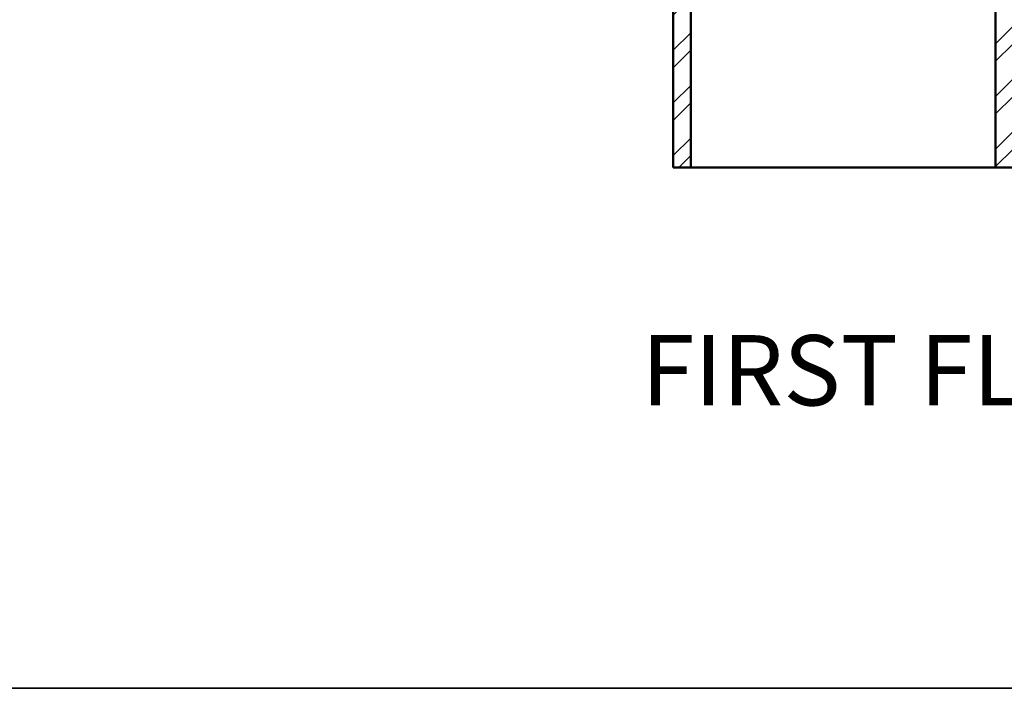
# Model space of a CAD drawing. Units: inches. Extents: x 963 to 2075, y 289 to 2657.
# Tile 3 of 98: x 1259 to 1511, y 1303 to 1474. Entities that reach past the tile are written whole.
import ezdxf

# ---------------------------------------------------------------- set-up
doc = ezdxf.new("R2010")
doc.units = ezdxf.units.IN
for name, color, linetype, lineweight in [('A-ANNO-TEXT', 7, 'Continuous', 25), ('A-ANNO-TTLB', 7, 'Continuous', 35), ('A-WALL', 7, 'Continuous', 50), ('A-WALL-PATT', 8, 'Continuous', 13)]:
    doc.layers.add(name, color=color, linetype=linetype, lineweight=lineweight)
doc.styles.get("Standard").update_dxf_attribs({"font": 'arial.ttf'})

msp = doc.modelspace()

# ---------------------------------------------------------------- hatches: boundary and pattern name
at = {"layer": 'A-WALL-PATT'}
h = msp.add_hatch(dxfattribs=at)
h.set_pattern_fill('ANSI32', color=256)
h.paths.add_polyline_path([(1296.92, 2558.32), (1203.92, 2558.32), (1203.92, 2493.82), (1191.53, 2493.82), (1191.53, 2489.32), (1211.06, 2489.32), (1211.06, 2492.02), (1211.06, 2493.82), (1208.42, 2493.82), (1208.42, 2553.82), (1292.42, 2553.82), (1292.42, 2538.86), (1296.92, 2538.86)])
h.paths.add_polyline_path([(1442.42, 2558.32), (1349.42, 2558.32), (1349.42, 2538.94), (1353.92, 2538.94), (1353.92, 2553.82), (1437.92, 2553.82), (1437.92, 2493.82), (1434.54, 2493.82), (1434.54, 2489.32), (1448.31, 2489.32), (1448.31, 2491.57), (1448.31, 2493.82), (1442.42, 2493.82)])
h.paths.add_polyline_path([(1415.55, 2491.57), (1415.55, 2493.82), (1340.94, 2493.82), (1340.94, 2489.32), (1371.92, 2489.32), (1371.92, 2378.32), (1367.6, 2378.32), (1367.6, 2373.82), (1371.92, 2373.82), (1371.92, 2355.19), (1376.42, 2355.19), (1376.42, 2489.32), (1415.55, 2489.32)])
h.paths.add_polyline_path([(1304.94, 2491.57), (1304.94, 2493.82), (1296.92, 2493.82), (1296.92, 2514.86), (1292.42, 2514.86), (1292.42, 2493.82), (1232.81, 2493.82), (1232.81, 2489.32), (1256.42, 2489.32), (1256.42, 2327.32), (1253.71, 2327.32), (1253.71, 2322.82), (1328.42, 2322.82), (1328.42, 2331.15), (1323.92, 2331.15), (1323.92, 2327.32), (1260.92, 2327.32), (1260.92, 2373.82), (1323.92, 2373.82), (1323.92, 2357.81), (1328.42, 2357.81), (1328.42, 2373.82), (1346.01, 2373.82), (1346.01, 2376.07), (1346.01, 2378.32), (1260.92, 2378.32), (1260.92, 2489.32), (1304.94, 2489.32)])
h.paths.add_polyline_path([(1226.65, 2327.32), (1124.42, 2327.32), (1124.42, 2347.45), (1119.92, 2347.45), (1119.92, 2322.82), (1163.42, 2322.82), (1163.42, 2305.43), (1165.67, 2305.43), (1167.92, 2305.43), (1167.92, 2322.82), (1226.65, 2322.82), (1226.65, 2325.07)])
h.paths.add_polyline_path([(1095.92, 2489.32), (1124.42, 2489.32), (1131.53, 2489.32), (1131.53, 2491.57), (1131.53, 2493.82), (1119.92, 2493.82), (1091.42, 2493.82), (1091.42, 2417.32), (1095.92, 2417.32), (1119.92, 2417.32), (1119.92, 2407.45), (1124.42, 2407.45), (1124.42, 2421.82), (1095.92, 2421.82)])
h.paths.add_polyline_path([(1512.92, 2558.32), (1508.42, 2558.32), (1508.42, 2493.82), (1503.4, 2493.82), (1503.4, 2489.32), (1508.42, 2489.32), (1508.42, 2327.32), (1376.42, 2327.32), (1376.42, 2330.27), (1371.92, 2330.27), (1371.92, 2298.74), (1376.42, 2298.74), (1376.42, 2322.82), (1508.42, 2322.82), (1508.42, 2165.32), (1504.26, 2165.32), (1504.26, 2160.82), (1508.42, 2160.82), (1508.42, 2108.32), (1512.92, 2108.32), (1512.92, 2160.82), (1516.18, 2160.82), (1516.18, 2163.07), (1516.18, 2165.32), (1512.92, 2165.32), (1512.92, 2322.82), (1644.92, 2322.82), (1644.92, 2298.74), (1649.42, 2298.74), (1649.42, 2322.82), (1649.42, 2330.94), (1647.17, 2330.94), (1644.92, 2330.94), (1644.92, 2327.32), (1512.92, 2327.32), (1512.92, 2489.32), (1516.76, 2489.32), (1516.76, 2491.57), (1516.76, 2493.82), (1512.92, 2493.82)])
h.paths.add_polyline_path([(1671.92, 2558.32), (1578.92, 2558.32), (1578.92, 2493.82), (1573.53, 2493.82), (1573.53, 2489.32), (1586.54, 2489.32), (1586.54, 2491.57), (1586.54, 2493.82), (1583.42, 2493.82), (1583.42, 2553.82), (1667.42, 2553.82), (1667.42, 2541.11), (1671.92, 2541.11)])
h.paths.add_polyline_path([(1681.26, 2493.82), (1671.92, 2493.82), (1671.92, 2517.11), (1667.42, 2517.11), (1667.42, 2493.82), (1610.22, 2493.82), (1610.22, 2489.32), (1644.92, 2489.32), (1644.92, 2357.87), (1649.42, 2357.87), (1649.42, 2373.82), (1652.2, 2373.82), (1652.2, 2375.83), (1652.2, 2378.32), (1649.42, 2378.32), (1649.42, 2489.32), (1681.26, 2489.32), (1681.26, 2491.57)])
h.paths.add_polyline_path([(1821.92, 2558.32), (1728.92, 2558.32), (1728.92, 2541), (1733.42, 2541), (1733.42, 2553.82), (1817.42, 2553.82), (1817.42, 2493.82), (1813.51, 2493.82), (1813.51, 2489.32), (1830.08, 2489.32), (1830.08, 2491.57), (1830.08, 2493.82), (1821.92, 2493.82)])
h.paths.add_polyline_path([(1794.24, 2493.82), (1717.26, 2493.82), (1717.26, 2489.32), (1760.42, 2489.32), (1760.42, 2378.32), (1674.4, 2378.32), (1674.4, 2373.82), (1692.92, 2373.82), (1692.92, 2356.95), (1697.42, 2356.95), (1697.42, 2373.82), (1760.42, 2373.82), (1760.42, 2327.32), (1697.42, 2327.32), (1697.42, 2333.34), (1692.92, 2333.34), (1692.92, 2322.82), (1768.04, 2322.82), (1768.04, 2325.07), (1768.04, 2327.32), (1764.92, 2327.32), (1764.92, 2489.32), (1794.24, 2489.32)])
h.paths.add_polyline_path([(1733.42, 2517), (1728.92, 2517), (1728.92, 2493.82), (1733.42, 2493.82)], flags=17)
h.paths.add_polyline_path([(1929.92, 2493.82), (1890.08, 2493.82), (1890.08, 2489.32), (1896.92, 2489.32), (1925.42, 2489.32), (1925.42, 2421.82), (1896.92, 2421.82), (1896.92, 2408.32), (1901.42, 2408.32), (1901.42, 2417.32), (1925.42, 2417.32), (1929.92, 2417.32)])
h.paths.add_polyline_path([(1901.42, 2348.32), (1896.92, 2348.32), (1896.92, 2327.32), (1800.42, 2327.32), (1800.42, 2322.82), (1853.42, 2322.82), (1853.42, 2309.45), (1857.92, 2309.45), (1857.92, 2322.82), (1901.42, 2322.82)])
h.paths.add_polyline_path([(1857.92, 2249.45), (1853.42, 2249.45), (1853.42, 2214.82), (1686.31, 2214.82), (1686.31, 2210.32), (1853.42, 2210.32), (1853.42, 2202.13), (1857.92, 2202.13), (1857.92, 2210.32)])
h.paths.add_polyline_path([(1857.92, 2142.13), (1853.42, 2142.13), (1853.42, 2115.42), (1841.42, 2115.42), (1841.42, 2088.53), (1841.42, 2046.95), (1845.92, 2046.95), (1845.92, 2110.92), (1905.92, 2110.92), (1905.92, 2092.52), (1910.42, 2092.52), (1910.42, 2115.42), (1857.92, 2115.42)])
h.paths.add_polyline_path([(1532.44, 1482.34), (1573.46, 1482.34), (1573.46, 1501), (1532.44, 1501)], flags=9)
h.paths.add_polyline_path([(1438.66, 1486.3), (1479.68, 1486.3), (1479.68, 1504.96), (1438.66, 1504.96)], flags=9)
h.paths.add_polyline_path([(1411.22, 1365.31), (1659.14, 1365.31), (1659.14, 1402.4), (1411.22, 1402.4)], flags=9)
h.paths.add_polyline_path([(1185.67, 2296.3), (1248.16, 2296.3), (1248.16, 2314.95), (1185.67, 2314.95)], flags=9)
h.paths.add_polyline_path([(1177.31, 2187.35), (1216.15, 2187.35), (1216.15, 2206.01), (1177.31, 2206.01)], flags=9)
h.paths.add_polyline_path([(1295.1, 1602.08), (1328.26, 1602.08), (1328.26, 1620.74), (1295.1, 1620.74)], flags=9)
h.paths.add_polyline_path([(1525.13, 2005.99), (1558.39, 2005.99), (1558.39, 2024.65), (1525.13, 2024.65)], flags=9)
h.paths.add_polyline_path([(1459.61, 1977.13), (1472.19, 1977.13), (1472.19, 1987.43), (1459.61, 1987.43)], flags=9)
h.paths.add_polyline_path([(1467.81, 2053.68), (1480.02, 2053.68), (1480.02, 2063.98), (1467.81, 2063.98)], flags=9)
h.paths.add_polyline_path([(1555.18, 2119.02), (1584.56, 2119.02), (1584.56, 2137.68), (1555.18, 2137.68)], flags=25)
h.paths.add_polyline_path([(1405.39, 2115.29), (1444.48, 2115.29), (1444.48, 2133.95), (1405.39, 2133.95)], flags=25)
h.paths.add_polyline_path([(1698.48, 2004.26), (1727.69, 2004.26), (1727.69, 2022.92), (1698.48, 2022.92)], flags=9)
h.paths.add_polyline_path([(1612.16, 1972.86), (1629.02, 1972.86), (1629.02, 1983.16), (1612.16, 1983.16)], flags=9)
h.paths.add_polyline_path([(1608.29, 2060.04), (1625.15, 2060.04), (1625.15, 2070.34), (1608.29, 2070.34)], flags=9)
h.paths.add_polyline_path([(1527.95, 1684.4), (1566.79, 1684.4), (1566.79, 1703.06), (1527.95, 1703.06)], flags=9)
h.paths.add_polyline_path([(1422.79, 1683.59), (1461.63, 1683.59), (1461.63, 1702.25), (1422.79, 1702.25)], flags=9)
h.paths.add_polyline_path([(1531.26, 1732.46), (1574.01, 1732.46), (1574.01, 1751.12), (1531.26, 1751.12)], flags=9)
h.paths.add_polyline_path([(1402.87, 1732.85), (1439.8, 1732.85), (1439.8, 1751.5), (1402.87, 1751.5)], flags=9)
h.paths.add_polyline_path([(1243.12, 1923.13), (1281.96, 1923.13), (1281.96, 1941.79), (1243.12, 1941.79)], flags=9)
h.paths.add_polyline_path([(1181.75, 1792.27), (1244.24, 1792.27), (1244.24, 1810.93), (1181.75, 1810.93)], flags=9)
h.paths.add_polyline_path([(1265.82, 1670.3), (1316.07, 1670.3), (1316.07, 1688.96), (1265.82, 1688.96)], flags=9)
h.paths.add_polyline_path([(1140.26, 1676.05), (1179.1, 1676.05), (1179.1, 1694.71), (1140.26, 1694.71)], flags=9)
h.paths.add_polyline_path([(1107.49, 1490.89), (1143.37, 1490.89), (1143.37, 1509.55), (1107.49, 1509.55)], flags=9)
h.paths.add_polyline_path([(1217.58, 1483.9), (1246.74, 1483.9), (1246.74, 1502.56), (1217.58, 1502.56)], flags=9)
h.paths.add_polyline_path([(1389.21, 1486.92), (1418.37, 1486.92), (1418.37, 1505.58), (1389.21, 1505.58)], flags=9)
h.paths.add_polyline_path([(1672.21, 1602.08), (1705.37, 1602.08), (1705.37, 1620.74), (1672.21, 1620.74)], flags=9)
h.paths.add_polyline_path([(1752.08, 1522.64), (1781.24, 1522.64), (1781.24, 1541.3), (1752.08, 1541.3)], flags=9)
h.paths.add_polyline_path([(1848.27, 1491.26), (1884.16, 1491.26), (1884.16, 1509.92), (1848.27, 1509.92)], flags=9)
h.paths.add_polyline_path([(1822.47, 1685.62), (1861.31, 1685.62), (1861.31, 1704.28), (1822.47, 1704.28)], flags=9)
h.paths.add_polyline_path([(1713.19, 1672.23), (1763.44, 1672.23), (1763.44, 1690.89), (1713.19, 1690.89)], flags=9)
h.paths.add_polyline_path([(1736.62, 1790.58), (1799.11, 1790.58), (1799.11, 1809.24), (1736.62, 1809.24)], flags=9)
h.paths.add_polyline_path([(1691.49, 1916.36), (1730.33, 1916.36), (1730.33, 1935.01), (1691.49, 1935.01)], flags=9)
h.paths.add_polyline_path([(1764.87, 1973.92), (1794.31, 1973.92), (1794.31, 1992.58), (1764.87, 1992.58)], flags=9)
h.paths.add_polyline_path([(1767.85, 2034.02), (1797.29, 2034.02), (1797.29, 2052.67), (1767.85, 2052.67)], flags=9)
h.paths.add_polyline_path([(1851.59, 2060.33), (1880.75, 2060.33), (1880.75, 2078.99), (1851.59, 2078.99)], flags=25)
h.paths.add_polyline_path([(1688.49, 2086.87), (1727.33, 2086.87), (1727.33, 2105.53), (1688.49, 2105.53)], flags=9)
h.paths.add_polyline_path([(1537.74, 2293.58), (1580.49, 2293.58), (1580.49, 2312.24), (1537.74, 2312.24)], flags=25)
h.paths.add_polyline_path([(1425.59, 2296.11), (1468.34, 2296.11), (1468.34, 2314.77), (1425.59, 2314.77)], flags=25)
h.paths.add_polyline_path([(1278.52, 2004.18), (1307.72, 2004.18), (1307.72, 2022.84), (1278.52, 2022.84)], flags=9)
h.paths.add_polyline_path([(1193.28, 1973.63), (1222.72, 1973.63), (1222.72, 1992.29), (1193.28, 1992.29)], flags=9)
h.paths.add_polyline_path([(1192.41, 2040.58), (1221.84, 2040.58), (1221.84, 2059.23), (1192.41, 2059.23)], flags=9)
h.paths.add_polyline_path([(1130.6, 1951.39), (1159.76, 1951.39), (1159.76, 1970.05), (1130.6, 1970.05)], flags=9)
h.paths.add_polyline_path([(1132.83, 2052.49), (1161.98, 2052.49), (1161.98, 2071.15), (1132.83, 2071.15)], flags=9)
h.paths.add_polyline_path([(1265.13, 2334.62), (1315.38, 2334.62), (1315.38, 2353.28), (1265.13, 2353.28)], flags=25)
h.paths.add_polyline_path([(1136.74, 2330.79), (1175.58, 2330.79), (1175.58, 2349.44), (1136.74, 2349.44)], flags=9)
h.paths.add_polyline_path([(1287.42, 2417.2), (1320.58, 2417.2), (1320.58, 2435.86), (1287.42, 2435.86)], flags=25)
h.paths.add_polyline_path([(1430.99, 2329.16), (1469.83, 2329.16), (1469.83, 2347.82), (1430.99, 2347.82)], flags=25)
h.paths.add_polyline_path([(1525.42, 2329.21), (1564.26, 2329.21), (1564.26, 2347.87), (1525.42, 2347.87)], flags=25)
h.paths.add_polyline_path([(1684.52, 2382.8), (1717.68, 2382.8), (1717.68, 2401.46), (1684.52, 2401.46)], flags=25)
h.paths.add_polyline_path([(1704.81, 2340.29), (1755.05, 2340.29), (1755.05, 2358.95), (1704.81, 2358.95)], flags=25)
h.paths.add_polyline_path([(1694.11, 2287.76), (1756.6, 2287.76), (1756.6, 2306.41), (1694.11, 2306.41)], flags=9)
h.paths.add_polyline_path([(1815.78, 2329.86), (1854.62, 2329.86), (1854.62, 2348.52), (1815.78, 2348.52)], flags=9)
h.paths.add_polyline_path([(1842.87, 2514.26), (1878.76, 2514.26), (1878.76, 2532.91), (1842.87, 2532.91)], flags=9)
h.paths.add_polyline_path([(1769.51, 2531.45), (1798.67, 2531.45), (1798.67, 2550.1), (1769.51, 2550.1)], flags=25)
h.paths.add_polyline_path([(1594.77, 2518.47), (1623.93, 2518.47), (1623.93, 2537.13), (1594.77, 2537.13)], flags=25)
h.paths.add_polyline_path([(1520.72, 2516.18), (1556.61, 2516.18), (1556.61, 2534.84), (1520.72, 2534.84)], flags=25)
h.paths.add_polyline_path([(1464.46, 2516.69), (1500.34, 2516.69), (1500.34, 2535.35), (1464.46, 2535.35)], flags=25)
h.paths.add_polyline_path([(1365.7, 2528.97), (1394.85, 2528.97), (1394.85, 2547.63), (1365.7, 2547.63)], flags=25)
h.paths.add_polyline_path([(1222.84, 2516.23), (1252, 2516.23), (1252, 2534.89), (1222.84, 2534.89)], flags=25)
h.paths.add_polyline_path([(1104.55, 2509.6), (1140.43, 2509.6), (1140.43, 2528.26), (1104.55, 2528.26)], flags=9)
h = msp.add_hatch(dxfattribs=at)
h.set_pattern_fill('ANSI32', color=256)
h.paths.add_polyline_path([(1335.97, 2212.57), (1335.97, 2214.82), (1167.92, 2214.82), (1167.92, 2245.43), (1163.42, 2245.43), (1163.42, 2210.32), (1163.42, 2194.81), (1167.92, 2194.81), (1167.92, 2210.32), (1335.97, 2210.32)])
h.paths.add_polyline_path([(1532.44, 1482.34), (1573.46, 1482.34), (1573.46, 1501), (1532.44, 1501)], flags=9)
h.paths.add_polyline_path([(1438.66, 1486.3), (1479.68, 1486.3), (1479.68, 1504.96), (1438.66, 1504.96)], flags=9)
h.paths.add_polyline_path([(1411.22, 1365.31), (1659.14, 1365.31), (1659.14, 1402.4), (1411.22, 1402.4)], flags=9)
h.paths.add_polyline_path([(1185.67, 2296.3), (1248.16, 2296.3), (1248.16, 2314.95), (1185.67, 2314.95)], flags=9)
h.paths.add_polyline_path([(1177.31, 2187.35), (1216.15, 2187.35), (1216.15, 2206.01), (1177.31, 2206.01)], flags=9)
h.paths.add_polyline_path([(1295.1, 1602.08), (1328.26, 1602.08), (1328.26, 1620.74), (1295.1, 1620.74)], flags=9)
h.paths.add_polyline_path([(1525.13, 2005.99), (1558.39, 2005.99), (1558.39, 2024.65), (1525.13, 2024.65)], flags=9)
h.paths.add_polyline_path([(1459.61, 1977.13), (1472.19, 1977.13), (1472.19, 1987.43), (1459.61, 1987.43)], flags=9)
h.paths.add_polyline_path([(1467.81, 2053.68), (1480.02, 2053.68), (1480.02, 2063.98), (1467.81, 2063.98)], flags=9)
h.paths.add_polyline_path([(1555.18, 2119.02), (1584.56, 2119.02), (1584.56, 2137.68), (1555.18, 2137.68)], flags=9)
h.paths.add_polyline_path([(1405.39, 2115.29), (1444.48, 2115.29), (1444.48, 2133.95), (1405.39, 2133.95)], flags=9)
h.paths.add_polyline_path([(1698.48, 2004.26), (1727.69, 2004.26), (1727.69, 2022.92), (1698.48, 2022.92)], flags=9)
h.paths.add_polyline_path([(1612.16, 1972.86), (1629.02, 1972.86), (1629.02, 1983.16), (1612.16, 1983.16)], flags=9)
h.paths.add_polyline_path([(1608.29, 2060.04), (1625.15, 2060.04), (1625.15, 2070.34), (1608.29, 2070.34)], flags=9)
h.paths.add_polyline_path([(1527.95, 1684.4), (1566.79, 1684.4), (1566.79, 1703.06), (1527.95, 1703.06)], flags=9)
h.paths.add_polyline_path([(1422.79, 1683.59), (1461.63, 1683.59), (1461.63, 1702.25), (1422.79, 1702.25)], flags=9)
h.paths.add_polyline_path([(1531.26, 1732.46), (1574.01, 1732.46), (1574.01, 1751.12), (1531.26, 1751.12)], flags=9)
h.paths.add_polyline_path([(1402.87, 1732.85), (1439.8, 1732.85), (1439.8, 1751.5), (1402.87, 1751.5)], flags=9)
h.paths.add_polyline_path([(1243.12, 1923.13), (1281.96, 1923.13), (1281.96, 1941.79), (1243.12, 1941.79)], flags=9)
h.paths.add_polyline_path([(1181.75, 1792.27), (1244.24, 1792.27), (1244.24, 1810.93), (1181.75, 1810.93)], flags=9)
h.paths.add_polyline_path([(1265.82, 1670.3), (1316.07, 1670.3), (1316.07, 1688.96), (1265.82, 1688.96)], flags=9)
h.paths.add_polyline_path([(1140.26, 1676.05), (1179.1, 1676.05), (1179.1, 1694.71), (1140.26, 1694.71)], flags=9)
h.paths.add_polyline_path([(1107.49, 1490.89), (1143.37, 1490.89), (1143.37, 1509.55), (1107.49, 1509.55)], flags=9)
h.paths.add_polyline_path([(1217.58, 1483.9), (1246.74, 1483.9), (1246.74, 1502.56), (1217.58, 1502.56)], flags=9)
h.paths.add_polyline_path([(1389.21, 1486.92), (1418.37, 1486.92), (1418.37, 1505.58), (1389.21, 1505.58)], flags=9)
h.paths.add_polyline_path([(1672.21, 1602.08), (1705.37, 1602.08), (1705.37, 1620.74), (1672.21, 1620.74)], flags=9)
h.paths.add_polyline_path([(1752.08, 1522.64), (1781.24, 1522.64), (1781.24, 1541.3), (1752.08, 1541.3)], flags=9)
h.paths.add_polyline_path([(1848.27, 1491.26), (1884.16, 1491.26), (1884.16, 1509.92), (1848.27, 1509.92)], flags=9)
h.paths.add_polyline_path([(1822.47, 1685.62), (1861.31, 1685.62), (1861.31, 1704.28), (1822.47, 1704.28)], flags=9)
h.paths.add_polyline_path([(1713.19, 1672.23), (1763.44, 1672.23), (1763.44, 1690.89), (1713.19, 1690.89)], flags=9)
h.paths.add_polyline_path([(1736.62, 1790.58), (1799.11, 1790.58), (1799.11, 1809.24), (1736.62, 1809.24)], flags=9)
h.paths.add_polyline_path([(1691.49, 1916.36), (1730.33, 1916.36), (1730.33, 1935.01), (1691.49, 1935.01)], flags=9)
h.paths.add_polyline_path([(1764.87, 1973.92), (1794.31, 1973.92), (1794.31, 1992.58), (1764.87, 1992.58)], flags=9)
h.paths.add_polyline_path([(1767.85, 2034.02), (1797.29, 2034.02), (1797.29, 2052.67), (1767.85, 2052.67)], flags=9)
h.paths.add_polyline_path([(1851.59, 2060.33), (1880.75, 2060.33), (1880.75, 2078.99), (1851.59, 2078.99)], flags=9)
h.paths.add_polyline_path([(1688.49, 2086.87), (1727.33, 2086.87), (1727.33, 2105.53), (1688.49, 2105.53)], flags=9)
h.paths.add_polyline_path([(1537.74, 2293.58), (1580.49, 2293.58), (1580.49, 2312.24), (1537.74, 2312.24)], flags=9)
h.paths.add_polyline_path([(1425.59, 2296.11), (1468.34, 2296.11), (1468.34, 2314.77), (1425.59, 2314.77)], flags=9)
h.paths.add_polyline_path([(1278.52, 2004.18), (1307.72, 2004.18), (1307.72, 2022.84), (1278.52, 2022.84)], flags=9)
h.paths.add_polyline_path([(1193.28, 1973.63), (1222.72, 1973.63), (1222.72, 1992.29), (1193.28, 1992.29)], flags=9)
h.paths.add_polyline_path([(1192.41, 2040.58), (1221.84, 2040.58), (1221.84, 2059.23), (1192.41, 2059.23)], flags=9)
h.paths.add_polyline_path([(1130.6, 1951.39), (1159.76, 1951.39), (1159.76, 1970.05), (1130.6, 1970.05)], flags=9)
h.paths.add_polyline_path([(1132.83, 2052.49), (1161.98, 2052.49), (1161.98, 2071.15), (1132.83, 2071.15)], flags=9)
h.paths.add_polyline_path([(1265.13, 2334.62), (1315.38, 2334.62), (1315.38, 2353.28), (1265.13, 2353.28)], flags=9)
h.paths.add_polyline_path([(1136.74, 2330.79), (1175.58, 2330.79), (1175.58, 2349.44), (1136.74, 2349.44)], flags=9)
h.paths.add_polyline_path([(1287.42, 2417.2), (1320.58, 2417.2), (1320.58, 2435.86), (1287.42, 2435.86)], flags=9)
h.paths.add_polyline_path([(1430.99, 2329.16), (1469.83, 2329.16), (1469.83, 2347.82), (1430.99, 2347.82)], flags=9)
h.paths.add_polyline_path([(1525.42, 2329.21), (1564.26, 2329.21), (1564.26, 2347.87), (1525.42, 2347.87)], flags=9)
h.paths.add_polyline_path([(1684.52, 2382.8), (1717.68, 2382.8), (1717.68, 2401.46), (1684.52, 2401.46)], flags=9)
h.paths.add_polyline_path([(1704.81, 2340.29), (1755.05, 2340.29), (1755.05, 2358.95), (1704.81, 2358.95)], flags=9)
h.paths.add_polyline_path([(1694.11, 2287.76), (1756.6, 2287.76), (1756.6, 2306.41), (1694.11, 2306.41)], flags=9)
h.paths.add_polyline_path([(1815.78, 2329.86), (1854.62, 2329.86), (1854.62, 2348.52), (1815.78, 2348.52)], flags=9)
h.paths.add_polyline_path([(1842.87, 2514.26), (1878.76, 2514.26), (1878.76, 2532.91), (1842.87, 2532.91)], flags=9)
h.paths.add_polyline_path([(1769.51, 2531.45), (1798.67, 2531.45), (1798.67, 2550.1), (1769.51, 2550.1)], flags=9)
h.paths.add_polyline_path([(1594.77, 2518.47), (1623.93, 2518.47), (1623.93, 2537.13), (1594.77, 2537.13)], flags=9)
h.paths.add_polyline_path([(1520.72, 2516.18), (1556.61, 2516.18), (1556.61, 2534.84), (1520.72, 2534.84)], flags=9)
h.paths.add_polyline_path([(1464.46, 2516.69), (1500.34, 2516.69), (1500.34, 2535.35), (1464.46, 2535.35)], flags=9)
h.paths.add_polyline_path([(1365.7, 2528.97), (1394.85, 2528.97), (1394.85, 2547.63), (1365.7, 2547.63)], flags=9)
h.paths.add_polyline_path([(1222.84, 2516.23), (1252, 2516.23), (1252, 2534.89), (1222.84, 2534.89)], flags=9)
h.paths.add_polyline_path([(1104.55, 2509.6), (1140.43, 2509.6), (1140.43, 2528.26), (1104.55, 2528.26)], flags=9)
h = msp.add_hatch(dxfattribs=at)
h.set_pattern_fill('ANSI32', color=256)
h.paths.add_polyline_path([(1473.61, 2163.07), (1473.61, 2165.32), (1376.42, 2165.32), (1376.42, 2227.98), (1371.92, 2227.98), (1371.92, 2214.82), (1368.41, 2214.82), (1368.41, 2210.32), (1371.92, 2210.32), (1371.92, 2160.82), (1395.92, 2160.82), (1395.92, 2090.32), (1217.34, 2090.32), (1217.34, 2085.82), (1395.92, 2085.82), (1458.92, 2085.82), (1458.92, 2108.32), (1454.42, 2108.32), (1454.42, 2090.32), (1400.42, 2090.32), (1400.42, 2160.82), (1473.61, 2160.82)])
h.paths.add_polyline_path([(1649.42, 2210.32), (1653.23, 2210.32), (1653.23, 2214.82), (1649.42, 2214.82), (1649.42, 2227.98), (1644.92, 2227.98), (1644.92, 2165.32), (1550.1, 2165.32), (1550.1, 2160.82), (1620.92, 2160.82), (1620.92, 2112.82), (1555.45, 2112.82), (1555.45, 2108.32), (1584.33, 2108.32), (1584.33, 2084.92), (1588.83, 2084.92), (1588.83, 2108.32), (1625.42, 2108.32), (1667.95, 2108.32), (1667.95, 2022.67), (1588.83, 2022.67), (1588.83, 2047.41), (1584.33, 2047.41), (1584.33, 1996), (1588.83, 1996), (1588.83, 2018.32), (1667.95, 2018.17), (1667.95, 1928.32), (1625.42, 1928.32), (1625.42, 1923.82), (1672.45, 1923.82), (1672.45, 1928.32), (1672.45, 1946.66), (1785.45, 1946.66), (1785.45, 1951.16), (1743.03, 1951.16), (1743.03, 2017.92), (1841.42, 2017.92), (1841.42, 2014.77), (1845.92, 2014.77), (1845.92, 2017.92), (1905.92, 2017.92), (1905.92, 1987.51), (1910.42, 1987.51), (1910.42, 2022.42), (1910.42, 2068.52), (1905.92, 2068.52), (1905.92, 2022.42), (1845.92, 2022.42), (1845.92, 2025.85), (1843.67, 2025.85), (1841.42, 2025.85), (1841.42, 2022.42), (1743.03, 2022.42), (1743.03, 2084.03), (1768.45, 2084.03), (1785.45, 2084.03), (1785.45, 2088.53), (1672.45, 2088.53), (1672.45, 2112.82), (1667.95, 2112.82), (1625.42, 2112.82), (1625.42, 2160.82), (1649.42, 2160.82)])
h.paths.add_polyline_path([(1672.45, 2084.03), (1738.53, 2084.03), (1738.53, 1951.16), (1672.45, 1951.16)], flags=16)
h.paths.add_polyline_path([(1672.45, 2084.03), (1738.53, 2084.03), (1705.49, 2017.6)], flags=0)
h.paths.add_polyline_path([(1262.77, 2085.82), (1258.27, 2085.82), (1258.27, 2023.28), (1184.42, 2023.28), (1184.42, 2018.78), (1258.27, 2018.78), (1258.27, 1950.82), (1262.77, 1950.82)])
h.paths.add_polyline_path([(1312.27, 2085.82), (1307.77, 2085.82), (1307.77, 1950.82), (1312.27, 1950.82)])
h.paths.add_polyline_path([(1458.92, 1950.82), (1395.92, 1950.82), (1216.57, 1950.82), (1216.57, 1946.32), (1346.42, 1946.32), (1395.92, 1946.32), (1395.92, 1875.82), (1371.92, 1875.82), (1371.92, 1826.32), (1368.93, 1826.32), (1368.93, 1821.82), (1371.92, 1821.82), (1371.92, 1813.62), (1376.42, 1813.62), (1376.42, 1871.32), (1474.5, 1871.32), (1474.5, 1873.57), (1474.5, 1875.82), (1400.42, 1875.82), (1400.42, 1946.32), (1454.42, 1946.32), (1454.42, 1928.32), (1458.92, 1928.32)])
h.paths.add_polyline_path([(1184.42, 2120.78), (1167.92, 2120.78), (1167.92, 2134.81), (1165.67, 2134.81), (1163.42, 2134.81), (1163.42, 2120.78), (1119.92, 2120.78), (1119.92, 2098.1), (1124.42, 2098.1), (1124.42, 2116.28), (1167.92, 2116.28), (1179.92, 2116.28), (1179.92, 2045.92), (1184.42, 2045.92), (1184.42, 2090.32), (1184.42, 2116.28)])
h.paths.add_polyline_path([(1124.42, 2018.78), (1179.92, 2018.78), (1179.92, 2016.29), (1184.42, 2016.29), (1184.42, 2023.28), (1184.42, 2026.59), (1182.17, 2026.59), (1179.92, 2026.59), (1179.92, 2023.28), (1124.42, 2023.28), (1124.42, 2074.1), (1119.92, 2074.1), (1119.92, 2018.78), (1119.92, 1979.63), (1124.42, 1979.63)])
h.paths.add_polyline_path([(1184.42, 1925.78), (1184.42, 1946.32), (1184.42, 1996.07), (1182.17, 1996.07), (1179.92, 1996.07), (1179.92, 1925.78), (1124.42, 1925.78), (1124.42, 1955.63), (1119.92, 1955.5), (1119.92, 1921.28), (1158.92, 1921.28), (1158.92, 1909.98), (1163.42, 1909.98), (1163.42, 1921.28), (1184.42, 1921.28)])
h.paths.add_polyline_path([(1341.45, 1826.32), (1163.42, 1826.32), (1163.42, 1849.98), (1158.92, 1849.98), (1158.92, 1821.82), (1158.92, 1804.03), (1163.42, 1804.03), (1163.42, 1821.82), (1341.45, 1821.82)])
h.paths.add_polyline_path([(1222.98, 1713.82), (1163.42, 1713.82), (1163.42, 1744.03), (1161.17, 1744.03), (1158.92, 1744.03), (1158.92, 1713.82), (1119.92, 1713.82), (1119.92, 1694.65), (1124.42, 1694.65), (1124.42, 1709.32), (1158.92, 1709.32), (1222.98, 1709.32)])
h.paths.add_polyline_path([(1328.42, 1713.82), (1252.04, 1713.82), (1252.04, 1711.57), (1252.04, 1709.32), (1256.42, 1709.32), (1256.42, 1547.32), (1232.94, 1547.32), (1232.94, 1545.07), (1232.94, 1542.82), (1292.42, 1542.82), (1292.42, 1527.63), (1296.92, 1527.63), (1296.92, 1542.82), (1299.46, 1542.82), (1299.46, 1547.32), (1260.92, 1547.32), (1260.92, 1658.32), (1343.66, 1658.32), (1343.66, 1660.57), (1343.66, 1662.82), (1328.42, 1662.82), (1328.42, 1676.59), (1327.4, 1676.59), (1323.92, 1676.59), (1323.92, 1662.82), (1260.92, 1662.82), (1260.92, 1709.32), (1323.92, 1709.32), (1323.92, 1699.85), (1328.42, 1699.85)])
h.paths.add_polyline_path([(1649.42, 1875.82), (1625.42, 1875.82), (1625.42, 1928.32), (1620.92, 1928.32), (1588.83, 1928.32), (1588.83, 1950.59), (1584.33, 1950.59), (1584.33, 1928.32), (1555.45, 1928.32), (1555.45, 1923.82), (1620.92, 1923.82), (1620.92, 1875.82), (1548.95, 1875.82), (1548.95, 1873.57), (1548.95, 1871.32), (1644.92, 1871.32), (1644.92, 1813.62), (1649.42, 1813.62), (1649.42, 1821.82), (1652.04, 1821.82), (1652.04, 1824.07), (1652.04, 1826.32), (1649.42, 1826.32)])
h.paths.add_polyline_path([(1512.92, 1871.32), (1516.48, 1871.32), (1516.48, 1875.82), (1512.92, 1875.82), (1512.92, 1923.82), (1512.92, 1928.32), (1512.92, 1930.83), (1508.42, 1930.83), (1508.42, 1875.82), (1504.41, 1875.82), (1504.41, 1871.32), (1508.42, 1871.32), (1508.42, 1713.82), (1376.42, 1713.82), (1376.42, 1743.32), (1371.92, 1743.32), (1371.92, 1709.32), (1371.92, 1706.01), (1376.42, 1706.01), (1376.42, 1709.32), (1508.42, 1709.32), (1508.42, 1547.32), (1501.87, 1547.32), (1501.87, 1542.82), (1508.42, 1542.82), (1508.42, 1482.82), (1508.42, 1436.32), (1512.92, 1436.32), (1512.92, 1542.82), (1519.32, 1542.82), (1519.32, 1545.07), (1519.32, 1547.32), (1512.92, 1547.32), (1512.92, 1709.32), (1644.92, 1709.32), (1644.92, 1707.55), (1649.42, 1707.55), (1649.42, 1709.32), (1649.42, 1743.32), (1644.92, 1743.32), (1644.92, 1713.82), (1512.92, 1713.82)])
h.paths.add_polyline_path([(1129.88, 1545.07), (1129.88, 1547.32), (1124.42, 1547.32), (1095.92, 1547.32), (1095.92, 1614.82), (1124.42, 1614.82), (1124.42, 1619.32), (1095.92, 1619.32), (1091.42, 1619.32), (1091.42, 1542.82), (1095.92, 1542.82), (1119.92, 1542.82), (1129.88, 1542.82)])
h.paths.add_polyline_path([(1208.42, 1542.82), (1211.74, 1542.82), (1211.74, 1547.32), (1198.85, 1547.32), (1198.85, 1542.82), (1203.92, 1542.82), (1203.92, 1478.32), (1208.42, 1478.32), (1296.92, 1478.32), (1296.92, 1503.63), (1292.42, 1503.63), (1292.42, 1482.82), (1208.42, 1482.82)])
h.paths.add_polyline_path([(1430.42, 1542.82), (1435.7, 1542.82), (1435.7, 1545.07), (1435.7, 1547.32), (1422.66, 1547.32), (1422.66, 1545.07), (1422.66, 1542.82), (1425.92, 1542.82), (1425.92, 1482.86), (1341.92, 1482.86), (1341.92, 1502.73), (1337.42, 1502.73), (1337.42, 1478.36), (1425.92, 1478.36), (1425.92, 1440.82), (1425.92, 1436.32), (1430.42, 1436.32)])
h.paths.add_polyline_path([(1698.48, 2004.26), (1727.69, 2004.26), (1727.69, 2022.92), (1698.48, 2022.92)], flags=8)

# ---------------------------------------------------------------- linework, layer by layer
at = {"layer": 'A-ANNO-TTLB'}
msp.add_lwpolyline([(962.81, 2657.49), (2074.6, 2657.49), (2074.6, 1303.08), (962.81, 1303.08)], close=True, dxfattribs=at)
at = {"layer": 'A-WALL'}
for p, q in [((1430.42, 1436.32), (1430.42, 1542.82)), ((1508.42, 1436.32), (1508.42, 1482.82)), ((1425.92, 1478.36), (1425.92, 1440.82)), ((1425.92, 1440.82), (1425.92, 1436.32)), ((1425.92, 1436.32), (1508.42, 1436.32)), ((1512.92, 1436.32), (1508.42, 1436.32))]:
    msp.add_line(p, q, dxfattribs=at)

# ---------------------------------------------------------------- texts
at = {"layer": 'A-ANNO-TEXT', "insert": (1417.78, 1393.46), "char_height": 18, "attachment_point": 1}
msp.add_mtext_dynamic_manual_height_columns('FIRST FLOOR PLAN ', width=783.3157, gutter_width=12.5, heights=[0], dxfattribs=at)

doc.saveas('drawing.dxf')
